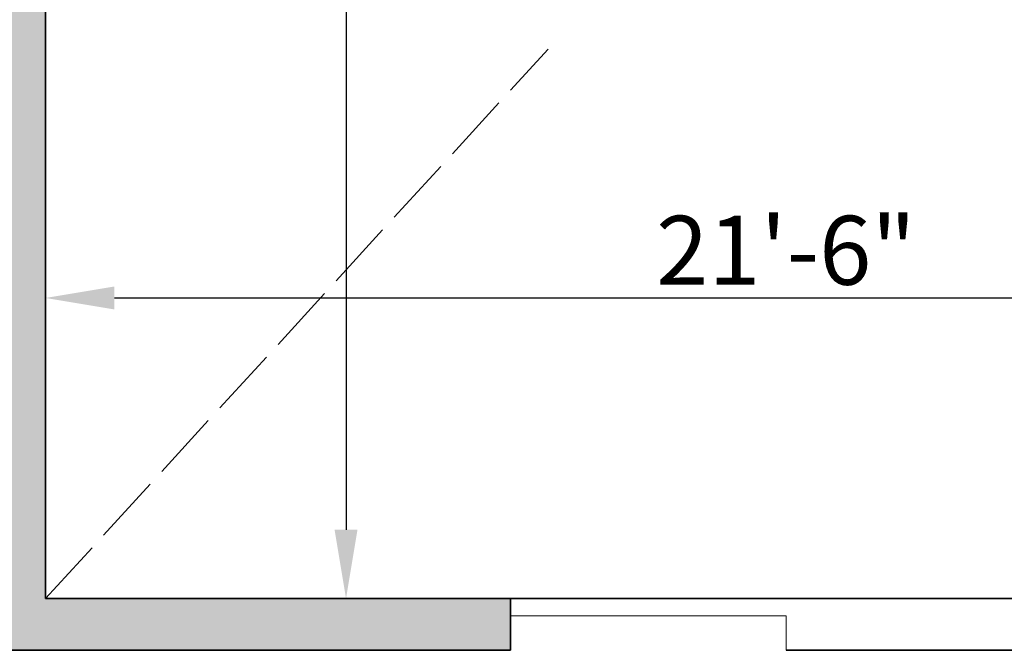
# Model space of a CAD drawing. Units: inches. Extents: x 2083 to 3317, y 1141 to 2115.
# Tile 108 of 256: x 2600 to 2772, y 1412 to 1522. Entities that reach past the tile are written whole.
import ezdxf

# ---------------------------------------------------------------- set-up
doc = ezdxf.new("R2010")
doc.units = ezdxf.units.IN
doc.linetypes.add('ACAD_ISO02W100', pattern=[15, 12, -3])
for name, color, linetype, lineweight in [('A-ANNO-DIMS', 2, 'Continuous', 18), ('A-FLOR-OPEN', 8, 'ACAD_ISO02W100', 13), ('A-GLAZ', 4, 'Continuous', 18), ('A-WALL', 7, 'Continuous', 35)]:
    doc.layers.add(name, color=color, linetype=linetype, lineweight=lineweight)
doc.layers.add('A-WALL-PATT', color=251, linetype='Continuous', lineweight=13, true_color=0x636466)
doc.styles.get("Standard").update_dxf_attribs({"font": 'arial.ttf'})
doc.dimstyles.new('ISO-25', dxfattribs={"dimtxt": 12, "dimasz": 12, "dimexe": 1.25, "dimexo": 0.625, "dimtad": 1, "dimlunit": 3, "dimtxsty": 'Standard', "dimcen": 2.5, "dimadec": 0, "dimazin": 0, "dimtfac": 1, "dimtmove": 0, "dimatfit": 3, "dimfxl": 1, "dimarcsym": 0})

# ---------------------------------------------------------------- blocks, each defined once
blk = doc.blocks.new('*D43')
at = {"layer": 'A-ANNO-DIMS', "color": 0, "lineweight": -2, "transparency": 16777216}
for p, q in [((2604.96, 1421.39), (2604.96, 1474.36)), ((2862.96, 1421.39), (2862.96, 1474.36)), ((2616.96, 1473.11), (2850.96, 1473.11))]:
    blk.add_line(p, q, dxfattribs=at)
at = {"layer": 'A-ANNO-DIMS', "color": 0, "transparency": 16777216}
for points in [[(2616.96, 1475.11), (2616.96, 1471.11), (2604.96, 1473.11)], [(2850.96, 1475.11), (2850.96, 1471.11), (2862.96, 1473.11)]]:
    blk.add_solid(points, dxfattribs=at)
at = {"layer": 'Defpoints', "color": 0, "transparency": 16777216}
for p in [(2862.96, 1473.11), (2604.96, 1420.76), (2862.96, 1420.76)]:
    blk.add_point(p, dxfattribs=at)
at = {"layer": 'A-ANNO-DIMS', "color": 0, "transparency": 16777216, "insert": (2733.96, 1479.86), "char_height": 12, "attachment_point": 5}
blk.add_mtext('21\'-6"', dxfattribs=at)
blk = doc.blocks.new('*D44')
at = {"layer": 'A-ANNO-DIMS', "color": 0, "lineweight": -2, "transparency": 16777216}
for p, q in [((2605.58, 1702.76), (2658.56, 1702.76)), ((2657.31, 1690.76), (2657.31, 1432.76)), ((2605.58, 1420.76), (2658.56, 1420.76))]:
    blk.add_line(p, q, dxfattribs=at)
at = {"layer": 'A-ANNO-DIMS', "color": 0, "transparency": 16777216}
for points in [[(2655.31, 1690.76), (2659.31, 1690.76), (2657.31, 1702.76)], [(2655.31, 1432.76), (2659.31, 1432.76), (2657.31, 1420.76)]]:
    blk.add_solid(points, dxfattribs=at)
at = {"layer": 'Defpoints', "color": 0, "transparency": 16777216}
for p in [(2604.96, 1702.76), (2604.96, 1420.76), (2657.31, 1420.76)]:
    blk.add_point(p, dxfattribs=at)
at = {"layer": 'A-ANNO-DIMS', "color": 0, "transparency": 16777216, "insert": (2650.55, 1561.76), "char_height": 12, "attachment_point": 5, "rotation": 90}
blk.add_mtext('23\'-6"', dxfattribs=at)

msp = doc.modelspace()

# ---------------------------------------------------------------- hatches: boundary and pattern name
at = {"layer": 'A-WALL-PATT'}
h = msp.add_hatch(color=256, dxfattribs=at)
h.dxf.hatch_style = 1
h.paths.add_polyline_path([(3126.96, 2020.761), (2748.96, 2020.761), (2604.96, 2020.761), (2226.96, 2020.761), (2226.96, 1702.761), (2466.96, 1702.761), (2466.96, 1582.761), (2418.96, 1582.761), (2418.96, 1477.761), (2226.96, 1477.761), (2226.96, 1263.261), (2544.96, 1263.261), (2544.96, 1411.761), (2604.96, 1411.761), (2685.96, 1411.761), (2685.96, 1420.761), (2604.96, 1420.761), (2604.96, 1573.761), (2604.96, 1702.761), (2604.96, 2011.761), (2748.96, 2011.761), (2748.96, 1702.761), (2862.96, 1702.761), (2862.96, 1621.761), (2871.96, 1621.761), (2871.96, 1702.761), (2883.96, 1702.761), (2883.96, 1706.939, -0.0264593), (2883.96, 1711.761), (2757.96, 1711.761), (2757.96, 1807.761), (2787.96, 1807.761), (2787.96, 1812.261), (2757.96, 1812.261), (2757.96, 2011.761), (2877.96, 2011.761), (2877.96, 1812.261), (2847.96, 1812.261), (2847.96, 1807.761), (2889.836, 1807.761), (2889.836, 1812.261), (2882.46, 1812.261), (2882.46, 2011.761), (3117.96, 2011.761), (3117.96, 1812.261), (2937.836, 1812.261), (2937.836, 1807.761), (2995.71, 1807.761), (2995.71, 1796.118), (3000.21, 1796.118), (3000.21, 1807.761), (3117.96, 1807.761), (3117.96, 1711.761), (3000.21, 1711.761), (3000.21, 1760.118), (2998.573, 1760.118, -0.020711), (2995.71, 1760.118), (2995.71, 1711.761), (2931.96, 1711.761), (2931.96, 1702.761), (3126.96, 1702.761)])
h.paths.add_polyline_path([(2471.46, 2011.761), (2471.46, 1810.011), (2462.717, 1810.011), (2462.717, 1805.511), (2505.96, 1805.511), (2505.96, 1810.011), (2475.96, 1810.011), (2475.96, 2011.761), (2595.96, 2011.761), (2595.96, 1810.011), (2565.96, 1810.011), (2565.96, 1805.511), (2595.96, 1805.511), (2595.96, 1711.761), (2235.96, 1711.761), (2235.96, 1805.511), (2353.71, 1805.511), (2353.71, 1796.054), (2358.21, 1796.054), (2358.21, 1805.511), (2414.717, 1805.511), (2414.717, 1810.011), (2235.96, 1810.011), (2235.96, 2011.761)], flags=16)
h.paths.add_polyline_path([(2270.205, 1994.61), (2270.205, 1970.61), (2246.205, 1970.61), (2246.205, 1994.61)], flags=0)
edge = h.paths.add_edge_path(flags=0)
edge.add_ellipse((2332.027, 1899.798), major_axis=(-3.043, 3.043), ratio=0.1682525, start_angle=-161.33217, end_angle=-156.30711, ccw=False)
edge.add_ellipse((2333.082, 1898.744), major_axis=(-1.055, 1.055), ratio=0.4535321, start_angle=-123.37102, end_angle=-94.15911)
edge = h.paths.add_edge_path(flags=0)
edge.add_ellipse((2332.027, 1968.876), major_axis=(3.043, 3.043), ratio=0.1682525, start_angle=18.66783, end_angle=23.69289)
edge.add_spline(control_points=[(2332.926, 1970.691), (2332.227, 1970.336), (2330.894, 1969.659), (2328.413, 1970.932), (2327.204, 1967.749), (2324.71, 1969.956), (2322.533, 1967.012), (2320.013, 1971.296), (2317.68, 1968.158), (2316.041, 1967.102), (2315.427, 1966.81)], knot_values=[0, 0, 0, 0, 2.2670587, 4.3245589, 6.6855835, 8.8786411, 11.121502, 14.300359, 17.7552837, 19.732645, 19.732645, 19.732645, 19.732645], degree=3, periodic=0)
edge.add_ellipse((2332.027, 1968.876), major_axis=(3.043, 3.043), ratio=0.1682525, start_angle=18.66783, end_angle=23.69289, ccw=False)
edge.add_ellipse((2333.082, 1969.931), major_axis=(1.055, 1.055), ratio=0.4535321, start_angle=56.62898, end_angle=85.84089, ccw=False)
edge = h.paths.add_edge_path(flags=0)
edge.add_spline(control_points=[(2296.428, 1967.988), (2293.628, 1965.336), (2287.704, 1959.727), (2299.744, 1949.996), (2294.533, 1935.669), (2290.573, 1920.604), (2293.394, 1909.974), (2296.185, 1904.967)], knot_values=[0.0991853, 0.0991853, 0.0991853, 0.0991853, 0.3453009, 0.6198217, 0.9826526, 1.3860932, 1.8105546, 1.8105546, 1.8105546, 1.8105546], degree=3, periodic=0)
edge.add_spline(control_points=[(2296.185, 1904.967), (2297.384, 1902.619), (2298.001, 1901.949), (2298.553, 1901.468)], knot_values=[0.0062457, 0.0062457, 0.0062457, 0.0062457, 0.0554759, 0.0554759, 0.0554759, 0.0554759], degree=3, periodic=0)
edge.add_spline(control_points=[(2298.553, 1901.468), (2297.259, 1900.923), (2295.225, 1900.232), (2293.06, 1900.614), (2292.101, 1900.788), (2292.09, 1900.791)], knot_values=[0.3128349, 0.3128349, 0.3128349, 0.3128349, 0.4017797, 0.4749867, 0.4759027, 0.4759027, 0.4759027, 0.4759027], degree=3, periodic=0)
edge.add_arc((2292.794, 1904.664), 3.937, 215.4209, 259.69818, ccw=False)
edge.add_spline(control_points=[(2289.585, 1902.382), (2289.477, 1902.535), (2289.368, 1902.688), (2289.261, 1902.841)], knot_values=[0.1028719, 0.1028719, 0.1028719, 0.1028719, 0.1168958, 0.1168958, 0.1168958, 0.1168958], degree=3, periodic=0)
edge.add_spline(control_points=[(2289.261, 1902.841), (2288.687, 1902.55), (2287.64, 1902.02), (2285.881, 1901.874), (2283.853, 1901.504), (2281.72, 1899.711), (2278.467, 1899.493), (2276.157, 1901.883), (2272.259, 1899.804), (2267.778, 1901.843), (2262.244, 1900.184), (2257.415, 1901.782), (2254.318, 1900.726), (2253.178, 1900.337)], knot_values=[0, 0, 0, 0, 1.9079767, 3.4771759, 5.261074, 7.9728515, 11.6802485, 13.7179214, 16.9395917, 22.789562, 27.5025027, 33.5952153, 37.1456181, 37.1456181, 37.1456181, 37.1456181], degree=3, periodic=0)
edge.add_line((2253.178, 1900.337), (2250.244, 1902.841))
edge.add_line((2250.244, 1902.841), (2250.244, 1965.833))
edge.add_line((2250.244, 1965.833), (2253.178, 1968.337))
edge.add_spline(control_points=[(2253.178, 1968.337), (2254.318, 1967.948), (2257.415, 1966.892), (2262.244, 1968.49), (2267.778, 1966.831), (2271.527, 1968.537), (2273.876, 1967.828), (2274.207, 1967.728)], knot_values=[0, 0, 0, 0, 0.0901802, 0.2449351, 0.3646438, 0.5132331, 0.5378548, 0.5378548, 0.5378548, 0.5378548], degree=3, periodic=0)
edge.add_arc((2274.353, 1963.793), 3.937, 72.05113, 92.12795, ccw=False)
edge.add_arc((2281.297, 1985.23), 18.596, 252.05113, 288.56572)
edge.add_arc((2292.317, 1956.029), 12.646, 71.02679, 113.77822, ccw=False)
edge = h.paths.add_edge_path(flags=0)
edge.add_spline(control_points=[(2274.899, 1951.856), (2275.066, 1951.617), (2275.233, 1951.377), (2275.398, 1951.136)], knot_values=[1.4099157, 1.4099157, 1.4099157, 1.4099157, 1.4315903, 1.4315903, 1.4315903, 1.4315903], degree=3, periodic=0)
edge.add_spline(control_points=[(2275.398, 1951.136), (2275.792, 1950.562), (2276.179, 1949.984), (2276.546, 1949.397)], knot_values=[1.3582378, 1.3582378, 1.3582378, 1.3582378, 1.4099157, 1.4099157, 1.4099157, 1.4099157], degree=3, periodic=0)
edge.add_line((2276.546, 1949.397), (2277.437, 1947.862))
edge.add_spline(control_points=[(2277.437, 1947.862), (2276.304, 1945.673), (2274.64, 1942.427), (2274.632, 1938.094), (2272.799, 1930.852), (2274.356, 1943.897), (2275.948, 1947.923), (2276.546, 1949.397)], knot_values=[0.0056315, 0.0056315, 0.0056315, 0.0056315, 0.1860139, 0.2660015, 0.3570872, 0.5963902, 0.7397317, 0.7397317, 0.7397317, 0.7397317], degree=3, periodic=0)
edge.add_spline(control_points=[(2276.546, 1949.397), (2276.179, 1949.984), (2275.792, 1950.562), (2275.398, 1951.136)], knot_values=[1.3582378, 1.3582378, 1.3582378, 1.3582378, 1.4099157, 1.4099157, 1.4099157, 1.4099157], degree=3, periodic=0)
edge.add_spline(control_points=[(2275.398, 1951.136), (2274.943, 1950.08), (2274.208, 1948.025), (2273.935, 1944.851), (2272.469, 1937.627), (2273.466, 1945.696), (2274.701, 1951.059), (2274.899, 1951.856)], knot_values=[0.1043639, 0.1043639, 0.1043639, 0.1043639, 0.1896363, 0.2696239, 0.3607096, 0.6000126, 0.6446217, 0.6446217, 0.6446217, 0.6446217], degree=3, periodic=0)
h.paths.add_polyline_path([(2269.168, 1963.128, -0.3575267), (2268.171, 1960.976, -0.0925607), (2268.171, 1939.436, -0.3575267), (2269.168, 1937.285, -0.3575267), (2267.016, 1938.282, -0.1647847), (2254.686, 1938.282, -0.3575267), (2252.534, 1937.285, -0.3575267), (2253.531, 1939.436, -0.0925607), (2253.531, 1960.976, -0.3575267), (2252.534, 1963.128, -0.3575267), (2254.686, 1962.131, -0.1647847), (2267.016, 1962.131, -0.3575267)], flags=0)
h.paths.add_polyline_path([(2248.874, 1967.802), (2248.874, 1957.028), (2249.458, 1957.028), (2249.458, 1911.647), (2248.874, 1911.647), (2248.874, 1900.873), (2246.512, 1900.873, 0.1973271), (2244.15, 1902.457), (2244.15, 1966.218, 0.1973271), (2246.512, 1967.802)], flags=0)
h.paths.add_polyline_path([(2269.168, 1931.389, -0.3575267), (2268.171, 1929.238, -0.0925607), (2268.171, 1907.698, -0.3575267), (2269.168, 1905.547, -0.3575267), (2267.016, 1906.544, -0.1647847), (2254.686, 1906.544, -0.3575267), (2252.534, 1905.547, -0.3575267), (2253.531, 1907.698, -0.0925607), (2253.531, 1929.238, -0.3575267), (2252.534, 1931.389, -0.3575267), (2254.686, 1930.392, -0.1647847), (2267.016, 1930.392, -0.3575267)], flags=0)
edge = h.paths.add_edge_path(flags=0)
edge.add_spline(control_points=[(2276.197, 1906.724), (2276.168, 1909.029), (2276.114, 1913.372), (2270.598, 1924.925), (2273.905, 1919.013), (2275.922, 1916.262), (2275.475, 1912.402), (2277.258, 1910.381), (2276.696, 1908.225), (2276.646, 1906.813), (2276.618, 1906.008)], knot_values=[0, 0, 0, 0, 8.6102597, 16.2212739, 18.8430575, 23.8048978, 27.4408283, 29.3561016, 31.2034776, 33.6506866, 33.6506866, 33.6506866, 33.6506866], degree=3, periodic=0)
edge.add_spline(control_points=[(2276.618, 1906.008), (2276.623, 1905.624), (2276.498, 1904.629), (2275.442, 1903.855), (2274.937, 1903.08), (2274.859, 1902.841)], knot_values=[0.1564884, 0.1564884, 0.1564884, 0.1564884, 0.1843975, 0.2313765, 0.2505985, 0.2505985, 0.2505985, 0.2505985], degree=3, periodic=0)
edge.add_line((2274.859, 1902.841), (2276.506, 1902.841))
edge.add_spline(control_points=[(2276.506, 1902.841), (2276.788, 1903.085), (2277.665, 1904.125), (2278.25, 1904.341), (2277.654, 1908.527), (2278.156, 1906.228), (2278.1, 1905.286), (2278.847, 1904.069), (2277.857, 1903.415), (2277.874, 1902.991), (2277.904, 1902.841)], knot_values=[0.0595743, 0.0595743, 0.0595743, 0.0595743, 0.0807529, 0.1037415, 0.1697201, 0.1760361, 0.2071372, 0.2404744, 0.2623409, 0.2736605, 0.2736605, 0.2736605, 0.2736605], degree=3, periodic=0)
edge.add_line((2277.904, 1902.841), (2280.03, 1902.841))
edge.add_spline(control_points=[(2280.03, 1902.841), (2279.888, 1903.088), (2279.499, 1903.982), (2280.152, 1905.939), (2278.104, 1909.658), (2279.762, 1907.185), (2280.328, 1904.875), (2280.485, 1903.49), (2281.463, 1903.249), (2281.758, 1902.936), (2281.834, 1902.841)], knot_values=[0.013856, 0.013856, 0.013856, 0.013856, 0.0348738, 0.0888667, 0.1078792, 0.1267378, 0.158714, 0.1937575, 0.2174868, 0.2267221, 0.2267221, 0.2267221, 0.2267221], degree=3, periodic=0)
edge.add_spline(control_points=[(2281.834, 1902.841), (2281.788, 1902.827), (2281.647, 1902.783), (2281.396, 1902.859), (2281.088, 1902.985), (2280.721, 1903.061), (2280.333, 1903.026), (2280.125, 1902.899), (2280.03, 1902.841)], knot_values=[0, 0, 0, 0, 0.1441304, 0.435517, 0.7492759, 1.1530457, 1.5483707, 1.878348, 1.878348, 1.878348, 1.878348], degree=3, periodic=0)
edge.add_line((2280.03, 1902.841), (2277.904, 1902.841))
edge.add_spline(control_points=[(2277.904, 1902.841), (2277.893, 1902.796), (2277.865, 1902.68), (2277.607, 1902.687), (2277.274, 1902.801), (2276.838, 1902.62), (2276.584, 1902.789), (2276.506, 1902.841)], knot_values=[0, 0, 0, 0, 0.1271885, 0.3261988, 0.6280094, 1.2435704, 1.5153306, 1.5153306, 1.5153306, 1.5153306], degree=3, periodic=0)
edge.add_line((2276.506, 1902.841), (2274.859, 1902.841))
edge.add_spline(control_points=[(2274.859, 1902.841), (2274.814, 1902.899), (2274.725, 1903.013), (2274.493, 1903.119), (2274.244, 1902.961), (2273.937, 1903.185), (2273.614, 1902.983), (2273.408, 1902.883), (2273.322, 1902.841)], knot_values=[0, 0, 0, 0, 0.2184302, 0.4369566, 0.6879766, 0.9903786, 1.3983955, 1.6918498, 1.6918498, 1.6918498, 1.6918498], degree=3, periodic=0)
edge.add_spline(control_points=[(2273.322, 1902.841), (2273.617, 1903.446), (2274.274, 1904.538), (2276.027, 1904.574), (2276.207, 1906.584), (2276.197, 1906.724)], knot_values=[0.0122268, 0.0122268, 0.0122268, 0.0122268, 0.0594721, 0.1062177, 0.134458, 0.134458, 0.134458, 0.134458], degree=3, periodic=0)
h.paths.add_polyline_path([(2270.776, 1897.79), (2270.776, 1873.79), (2246.776, 1873.79), (2246.776, 1897.79)], flags=0)
h.paths.add_polyline_path([(2353.71, 1760.005), (2353.71, 1760.054), (2358.21, 1760.054, -0.033729)], flags=0)
h.paths.add_polyline_path([(2321.819, 1737.529), (2341.995, 1737.529, -0.4142136), (2343.203, 1736.321), (2343.203, 1721.021, -0.4142136), (2341.995, 1719.813), (2321.819, 1719.813, -0.4142136), (2320.611, 1721.021), (2320.611, 1736.321, -0.4142136)], flags=0)
h.paths.add_polyline_path([(2324.235, 1736.321), (2339.579, 1736.321, -0.4142136), (2341.995, 1733.905), (2341.995, 1725.45, -0.4142136), (2339.579, 1723.034), (2333.681, 1723.034), (2333.845, 1722.045, -0.8706461), (2335.425, 1721.826, -0.767327), (2333.923, 1721.423), (2331.291, 1721.423, -0.767327), (2329.788, 1721.826, -0.8706461), (2331.368, 1722.045), (2331.533, 1723.034), (2324.235, 1723.034, -0.4142136), (2321.819, 1725.45), (2321.819, 1733.905, -0.4142136)], flags=0)
h.paths.add_polyline_path([(2570.484, 1928.615), (2589.684, 1928.615), (2590.169, 1928.615), (2590.169, 1904.993), (2570.484, 1904.993)], flags=0)
h.paths.add_polyline_path([(2574.447, 1927.264, -1), (2572.829, 1927.264, -1)], flags=0)
h.paths.add_polyline_path([(2573.09, 1926.941), (2573.925, 1927.776), (2574.148, 1927.553), (2573.313, 1926.718)], flags=0)
h.paths.add_polyline_path([(2578.779, 1919.73, -1), (2571.592, 1919.73, -1)], flags=0)
h.paths.add_polyline_path([(2578.385, 1919.73, -1), (2571.985, 1919.73, -1)], flags=0)
h.paths.add_polyline_path([(2331.596, 1729.476, -1), (2333.618, 1729.476, -1)], flags=0)
h.paths.add_polyline_path([(2578.034, 1927.264, -1), (2576.416, 1927.264, -1)], flags=0)
h.paths.add_polyline_path([(2576.689, 1927.531), (2576.912, 1927.754), (2577.747, 1926.919), (2577.524, 1926.696)], flags=0)
h.paths.add_polyline_path([(2578.139, 1909.86, -1), (2572.232, 1909.86, -1)], flags=0)
h.paths.add_polyline_path([(2577.745, 1909.86, -1), (2572.625, 1909.86, -1)], flags=0)
h.paths.add_polyline_path([(2583.798, 1927.264, -1), (2582.179, 1927.264, -1)], flags=0)
h.paths.add_polyline_path([(2582.719, 1927.754), (2583.554, 1926.919), (2583.331, 1926.696), (2582.496, 1927.531)], flags=0)
h.paths.add_polyline_path([(2582.496, 1927.531), (2582.719, 1927.754), (2583.554, 1926.919), (2583.331, 1926.696)], flags=0)
h.paths.add_polyline_path([(2587.739, 1920.53, -1), (2581.832, 1920.53, -1)], flags=0)
h.paths.add_polyline_path([(2587.345, 1920.53, -1), (2582.225, 1920.53, -1)], flags=0)
h.paths.add_polyline_path([(2587.385, 1927.264, -1), (2585.766, 1927.264, -1)], flags=0)
h.paths.add_polyline_path([(2586.082, 1926.98), (2586.917, 1927.815), (2587.14, 1927.593), (2586.305, 1926.758)], flags=0)
h.paths.add_polyline_path([(2588.379, 1910.66, -1), (2581.192, 1910.66, -1)], flags=0)
h.paths.add_polyline_path([(2587.985, 1910.66, -1), (2581.585, 1910.66, -1)], flags=0)
h.paths.add_polyline_path([(2417.168, 1729.478), (2437.344, 1729.478, -0.4142136), (2438.552, 1728.27), (2438.552, 1712.969, -0.4142136), (2437.344, 1711.761), (2417.168, 1711.761, -0.4142136), (2415.96, 1712.969), (2415.96, 1728.27, -0.4142136)], flags=0)
h.paths.add_polyline_path([(2419.584, 1728.27), (2434.928, 1728.27, -0.4142136), (2437.344, 1725.854), (2437.344, 1717.398, -0.4142136), (2434.928, 1714.983), (2429.029, 1714.983), (2429.194, 1713.994, -0.8706461), (2430.774, 1713.775, -0.767327), (2429.271, 1713.372), (2426.64, 1713.372, -0.767327), (2425.137, 1713.775, -0.8706461), (2426.717, 1713.994), (2426.882, 1714.983), (2419.584, 1714.983, -0.4142136), (2417.168, 1717.398), (2417.168, 1725.854, -0.4142136)], flags=0)
h.paths.add_polyline_path([(2419.584, 1728.27), (2434.928, 1728.27, -0.4142136), (2437.344, 1725.854), (2437.344, 1717.398, -0.4142136), (2434.928, 1714.983), (2429.029, 1714.983), (2428.358, 1719.009), (2427.553, 1719.009), (2426.882, 1714.983), (2419.584, 1714.983, -0.4142136), (2417.168, 1717.398), (2417.168, 1725.854, -0.4142136)], flags=0)
h.paths.add_polyline_path([(2426.944, 1721.425, -1), (2428.967, 1721.425, -1)], flags=0)
h.paths.add_polyline_path([(2475.96, 1702.761), (2595.96, 1702.761), (2595.96, 1582.761), (2475.96, 1582.761)], flags=16)
h.paths.add_polyline_path([(2427.96, 1573.761), (2595.96, 1573.761), (2595.96, 1468.761), (2595.96, 1420.761), (2384.46, 1420.761), (2384.46, 1468.761), (2427.96, 1468.761)], flags=16)
h.paths.add_polyline_path([(2379.96, 1468.761), (2379.96, 1420.761), (2235.96, 1420.761), (2235.96, 1468.761)], flags=16)
h.paths.add_polyline_path([(2317.816, 1466.696), (2337.992, 1466.696, -0.4142136), (2339.2, 1465.488), (2339.2, 1450.187, -0.4142136), (2337.992, 1448.979), (2317.816, 1448.979, -0.4142136), (2316.608, 1450.187), (2316.608, 1465.488, -0.4142136)], flags=0)
h.paths.add_polyline_path([(2320.232, 1465.488), (2335.576, 1465.488, -0.4142136), (2337.992, 1463.072), (2337.992, 1454.616, -0.4142136), (2335.576, 1452.2), (2329.677, 1452.2), (2329.842, 1451.212, -0.8706461), (2331.422, 1450.992, -0.767327), (2329.92, 1450.59), (2327.288, 1450.59, -0.767327), (2325.785, 1450.992, -0.8706461), (2327.365, 1451.212), (2327.53, 1452.2), (2320.232, 1452.2, -0.4142136), (2317.816, 1454.616), (2317.816, 1463.072, -0.4142136)], flags=0)
h.paths.add_polyline_path([(2320.232, 1465.488), (2335.576, 1465.488, -0.4142136), (2337.992, 1463.072), (2337.992, 1454.616, -0.4142136), (2335.576, 1452.2), (2329.677, 1452.2), (2329.006, 1456.227), (2328.201, 1456.227), (2327.53, 1452.2), (2320.232, 1452.2, -0.4142136), (2317.816, 1454.616), (2317.816, 1463.072, -0.4142136)], flags=0)
h.paths.add_polyline_path([(2327.593, 1458.643, -1), (2329.615, 1458.643, -1)], flags=0)
h.paths.add_polyline_path([(2244.412, 1433.34), (2241.921, 1433.34, -0.4142136), (2240.018, 1435.244), (2240.018, 1440.953, -0.4142105), (2241.921, 1442.856), (2244.412, 1442.856, -1.9764724)], flags=0)
h.paths.add_polyline_path([(2245.357, 1434.398, -0.4142136), (2245.357, 1441.799, -2.1440985)], flags=0)
h.paths.add_polyline_path([(2535.96, 1416.261), (2535.96, 1272.261), (2235.96, 1272.261), (2235.96, 1416.261)], flags=16)
h.paths.add_polyline_path([(2260.12, 1384.293), (2260.12, 1362.039), (2237.865, 1362.039), (2237.865, 1384.293)], flags=0)
edge = h.paths.add_edge_path(flags=0)
edge.add_line((2318.252, 1362.093), (2318.146, 1362.001))
edge.add_ellipse((2317.445, 1360.431), major_axis=(2.822, 2.822), ratio=0.1682525, start_angle=18.66783, end_angle=20.94813, ccw=False)
edge.add_ellipse((2318.423, 1361.409), major_axis=(0.978, 0.978), ratio=0.4535321, start_angle=56.62898, end_angle=70.2262, ccw=False)
edge = h.paths.add_edge_path(flags=0)
edge.add_line((2319.107, 1295.571), (2319.015, 1295.677))
edge.add_ellipse((2317.445, 1296.378), major_axis=(-2.822, 2.822), ratio=0.1682525, start_angle=-161.33217, end_angle=-159.05187, ccw=False)
edge.add_ellipse((2318.423, 1295.4), major_axis=(-0.978, 0.978), ratio=0.4535321, start_angle=-123.37102, end_angle=-109.7738)
edge = h.paths.add_edge_path(flags=0)
edge.add_spline(control_points=[(2284.21, 1301.17), (2284.581, 1300.445), (2284.891, 1299.892), (2285.16, 1299.461)], knot_values=[0.0390658, 0.0390658, 0.0390658, 0.0390658, 0.0554759, 0.0554759, 0.0554759, 0.0554759], degree=3, periodic=0)
edge.add_line((2285.16, 1299.461), (2284.21, 1301.17))
edge = h.paths.add_edge_path(flags=0)
edge.add_line((2280.412, 1297.298), (2283.37, 1297.036))
edge.add_line((2283.37, 1297.036), (2286.406, 1297.926))
edge.add_spline(control_points=[(2286.406, 1297.926), (2285.305, 1297.463), (2284.345, 1297.129), (2283.37, 1297.036)], knot_values=[0.3943688, 0.3943688, 0.3943688, 0.3943688, 0.4759027, 0.4759027, 0.4759027, 0.4759027], degree=3, periodic=0)
edge.add_spline(control_points=[(2283.37, 1297.036), (2283.281, 1297.028), (2282.316, 1296.957), (2281.313, 1297.134), (2280.423, 1297.296), (2280.412, 1297.298)], knot_values=[0.3128349, 0.3128349, 0.3128349, 0.3128349, 0.3202458, 0.3934528, 0.3943688, 0.3943688, 0.3943688, 0.3943688], degree=3, periodic=0)
edge = h.paths.add_edge_path(flags=0)
edge.add_line((2284.436, 1359.607), (2280.446, 1355.328))
edge.add_line((2280.446, 1355.328), (2279.58, 1351.018))
edge.add_line((2279.58, 1351.018), (2282.413, 1346.58))
edge.add_spline(control_points=[(2282.413, 1346.58), (2283.153, 1345.589), (2284.253, 1344.029), (2284.801, 1342.387), (2284.935, 1341.806)], knot_values=[1.2400982, 1.2400982, 1.2400982, 1.2400982, 1.3328922, 1.3827123, 1.3827123, 1.3827123, 1.3827123], degree=3, periodic=0)
edge.add_spline(control_points=[(2284.935, 1341.806), (2285.319, 1340.141), (2285.233, 1338.409), (2284.91, 1336.654)], knot_values=[1.0974841, 1.0974841, 1.0974841, 1.0974841, 1.2400982, 1.2400982, 1.2400982, 1.2400982], degree=3, periodic=0)
edge.add_spline(control_points=[(2284.91, 1336.654), (2284.587, 1334.899), (2284.027, 1333.12), (2283.463, 1331.361)], knot_values=[0.9548699, 0.9548699, 0.9548699, 0.9548699, 1.0974841, 1.0974841, 1.0974841, 1.0974841], degree=3, periodic=0)
edge.add_line((2283.463, 1331.361), (2281.89, 1326.153))
edge.add_line((2281.89, 1326.153), (2280.756, 1321.056))
edge.add_line((2280.756, 1321.056), (2280.299, 1316.002))
edge.add_line((2280.299, 1316.002), (2280.716, 1310.95))
edge.add_line((2280.716, 1310.95), (2282.028, 1305.972))
edge.add_line((2282.028, 1305.972), (2284.21, 1301.17))
edge.add_spline(control_points=[(2284.21, 1301.17), (2283.341, 1302.73), (2282.612, 1304.336), (2282.028, 1305.972)], knot_values=[0.0991853, 0.0991853, 0.0991853, 0.0991853, 0.2417994, 0.2417994, 0.2417994, 0.2417994], degree=3, periodic=0)
edge.add_spline(control_points=[(2282.028, 1305.972), (2281.444, 1307.608), (2281.005, 1309.273), (2280.716, 1310.95)], knot_values=[0.2417994, 0.2417994, 0.2417994, 0.2417994, 0.3844135, 0.3844135, 0.3844135, 0.3844135], degree=3, periodic=0)
edge.add_spline(control_points=[(2280.716, 1310.95), (2280.433, 1312.588), (2280.289, 1314.277), (2280.299, 1315.962), (2280.299, 1316.002)], knot_values=[0.3844135, 0.3844135, 0.3844135, 0.3844135, 0.5236467, 0.5270276, 0.5270276, 0.5270276, 0.5270276], degree=3, periodic=0)
edge.add_spline(control_points=[(2280.299, 1316.002), (2280.312, 1317.687), (2280.478, 1319.368), (2280.756, 1321.056)], knot_values=[0.5270276, 0.5270276, 0.5270276, 0.5270276, 0.6696417, 0.6696417, 0.6696417, 0.6696417], degree=3, periodic=0)
edge.add_spline(control_points=[(2280.756, 1321.056), (2281.035, 1322.744), (2281.426, 1324.44), (2281.89, 1326.153)], knot_values=[0.6696417, 0.6696417, 0.6696417, 0.6696417, 0.8122558, 0.8122558, 0.8122558, 0.8122558], degree=3, periodic=0)
edge.add_spline(control_points=[(2281.89, 1326.153), (2282.264, 1327.533), (2282.788, 1329.262), (2283.353, 1331.018), (2283.463, 1331.361)], knot_values=[0.8122558, 0.8122558, 0.8122558, 0.8122558, 0.9270873, 0.9548699, 0.9548699, 0.9548699, 0.9548699], degree=3, periodic=0)
edge.add_line((2283.463, 1331.361), (2284.91, 1336.654))
edge.add_line((2284.91, 1336.654), (2284.935, 1341.806))
edge.add_line((2284.935, 1341.806), (2282.413, 1346.58))
edge.add_spline(control_points=[(2282.413, 1346.58), (2281.275, 1348.104), (2280.078, 1349.57), (2279.58, 1351.018)], knot_values=[1.3827123, 1.3827123, 1.3827123, 1.3827123, 1.5253264, 1.5253264, 1.5253264, 1.5253264], degree=3, periodic=0)
edge.add_spline(control_points=[(2279.58, 1351.018), (2279.443, 1351.415), (2279.136, 1352.857), (2279.735, 1354.29), (2280.446, 1355.328)], knot_values=[1.5253264, 1.5253264, 1.5253264, 1.5253264, 1.564439, 1.6679405, 1.6679405, 1.6679405, 1.6679405], degree=3, periodic=0)
edge.add_spline(control_points=[(2280.446, 1355.328), (2281.426, 1356.758), (2282.931, 1358.183), (2284.436, 1359.607)], knot_values=[1.6679405, 1.6679405, 1.6679405, 1.6679405, 1.8105546, 1.8105546, 1.8105546, 1.8105546], degree=3, periodic=0)
edge.add_arc((2280.623, 1348.518), 11.726, 71.02679, 113.77822)
edge.add_arc((2270.405, 1375.595), 17.244, 252.05113, 288.56572, ccw=False)
edge.add_arc((2263.966, 1355.718), 3.651, 72.05113, 92.12795)
edge.add_arc((2263.966, 1355.718), 3.651, 92.12795, 177.98513)
edge.add_spline(control_points=[(2260.318, 1355.846), (2260.26, 1354.221), (2260.551, 1350.187), (2262.999, 1346.766), (2264.473, 1344.649)], knot_values=[1.4315903, 1.4315903, 1.4315903, 1.4315903, 1.5641438, 1.7706953, 1.7706953, 1.7706953, 1.7706953], degree=3, periodic=0)
edge.add_line((2264.473, 1344.649), (2264.936, 1343.983))
edge.add_spline(control_points=[(2263.801, 1340.248), (2263.843, 1340.514), (2264.067, 1341.756), (2264.513, 1343.002), (2264.935, 1343.981)], knot_values=[0.5365702, 0.5365702, 0.5365702, 0.5365702, 0.5593494, 0.6446217, 0.6446217, 0.6446217, 0.6446217], degree=3, periodic=0)
edge.add_spline(control_points=[(2264.935, 1343.981), (2265.118, 1343.715), (2265.299, 1343.448), (2265.477, 1343.179)], knot_values=[1.3840767, 1.3840767, 1.3840767, 1.3840767, 1.4099157, 1.4099157, 1.4099157, 1.4099157], degree=3, periodic=0)
edge.add_spline(control_points=[(2265.477, 1343.179), (2265.655, 1342.911), (2265.829, 1342.641), (2265.999, 1342.369)], knot_values=[1.3582378, 1.3582378, 1.3582378, 1.3582378, 1.3840767, 1.3840767, 1.3840767, 1.3840767], degree=3, periodic=0)
edge.add_line((2265.999, 1342.369), (2266.826, 1340.946))
edge.add_spline(control_points=[(2266.826, 1340.946), (2268.894, 1337.09), (2271.398, 1325.843), (2270.516, 1310.569), (2275.919, 1301.861), (2277.79, 1299.199)], knot_values=[0.1168958, 0.1168958, 0.1168958, 0.1168958, 0.4729873, 1.0509689, 1.3137934, 1.3137934, 1.3137934, 1.3137934], degree=3, periodic=0)
edge.add_spline(control_points=[(2277.79, 1299.199), (2277.839, 1299.128), (2277.889, 1299.057), (2277.94, 1298.987)], knot_values=[0.1098839, 0.1098839, 0.1098839, 0.1098839, 0.1168958, 0.1168958, 0.1168958, 0.1168958], degree=3, periodic=0)
edge.add_line((2277.94, 1298.987), (2277.789, 1299.199))
edge.add_spline(control_points=[(2277.789, 1299.199), (2277.257, 1298.929), (2276.286, 1298.438), (2275.039, 1298.334), (2274.383, 1298.239), (2274.215, 1298.209)], knot_values=[33.1218702, 33.1218702, 33.1218702, 33.1218702, 35.0290557, 36.5982549, 37.1448269, 37.1448269, 37.1448269, 37.1448269], degree=3, periodic=0)
edge.add_line((2274.215, 1298.209), (2273.073, 1297.893))
edge.add_spline(control_points=[(2273.073, 1297.893), (2272.323, 1297.58), (2271.039, 1296.511), (2269.248, 1296.226), (2268.423, 1296.375)], knot_values=[26.5325843, 26.5325843, 26.5325843, 26.5325843, 29.198919, 31.8391012, 31.8391012, 31.8391012, 31.8391012], degree=3, periodic=0)
edge.add_line((2268.423, 1296.375), (2263.879, 1297.458))
edge.add_spline(control_points=[(2263.879, 1297.458), (2263.556, 1297.359), (2261.86, 1296.839), (2260.239, 1297.282), (2258.933, 1297.516)], knot_values=[15.9195506, 15.9195506, 15.9195506, 15.9195506, 16.9395917, 21.2260675, 21.2260675, 21.2260675, 21.2260675], degree=3, periodic=0)
edge.add_line((2258.933, 1297.516), (2254.055, 1297.329))
edge.add_spline(control_points=[(2254.055, 1297.329), (2253.756, 1297.296), (2252.114, 1297.165), (2250.462, 1297.544), (2249.13, 1297.668)], knot_values=[5.3065169, 5.3065169, 5.3065169, 5.3065169, 6.2764352, 10.6130337, 10.6130337, 10.6130337, 10.6130337], degree=3, periodic=0)
edge.add_line((2249.13, 1297.668), (2244.332, 1296.878))
edge.add_line((2244.332, 1296.878), (2241.611, 1299.199))
edge.add_line((2241.611, 1299.199), (2241.611, 1357.609))
edge.add_line((2241.611, 1357.609), (2244.332, 1359.931))
edge.add_line((2244.332, 1359.931), (2252.729, 1359.543))
edge.add_spline(control_points=[(2252.729, 1359.543), (2252.871, 1359.546), (2253.306, 1359.548), (2253.74, 1359.514), (2254.032, 1359.482)], knot_values=[0.233291, 0.233291, 0.233291, 0.233291, 0.2449351, 0.2689274, 0.2689274, 0.2689274, 0.2689274], degree=3, periodic=0)
edge.add_line((2254.032, 1359.482), (2259.587, 1359.416))
edge.add_spline(control_points=[(2259.587, 1359.416), (2260.677, 1359.629), (2262.073, 1359.897), (2263.524, 1359.459), (2263.83, 1359.366)], knot_values=[0.4225164, 0.4225164, 0.4225164, 0.4225164, 0.5132331, 0.5378548, 0.5378548, 0.5378548, 0.5378548], degree=3, periodic=0)
edge.add_arc((2263.966, 1355.718), 3.651, 72.05113, 92.12795, ccw=False)
edge.add_arc((2270.405, 1375.595), 17.244, 252.05113, 288.56572)
edge.add_arc((2280.623, 1348.518), 11.726, 71.02679, 113.77822, ccw=False)
h.paths.add_polyline_path([(2240.341, 1359.435), (2240.341, 1349.444), (2240.882, 1349.444), (2240.882, 1307.365), (2240.341, 1307.365), (2240.341, 1297.374), (2238.15, 1297.374, 0.1973271), (2235.96, 1298.843), (2235.96, 1357.966, 0.1973271), (2238.15, 1359.435)], flags=0)
h.paths.add_polyline_path([(2259.158, 1355.101, -0.3575267), (2258.233, 1353.106, -0.0925607), (2258.233, 1333.133, -0.3575267), (2259.158, 1331.138, -0.3575267), (2257.163, 1332.062, -0.1647847), (2245.729, 1332.062, -0.3575267), (2243.735, 1331.138, -0.3575267), (2244.659, 1333.133, -0.0925607), (2244.659, 1353.106, -0.3575267), (2243.735, 1355.101, -0.3575267), (2245.729, 1354.176, -0.1647847), (2257.163, 1354.176, -0.3575267)], flags=0)
edge = h.paths.add_edge_path(flags=0)
edge.add_line((2265.999, 1342.369), (2266.826, 1340.946))
edge.add_line((2266.826, 1340.946), (2265.308, 1337.814))
edge.add_line((2265.308, 1337.814), (2264.358, 1334.653))
edge.add_line((2264.358, 1334.653), (2264.262, 1333.8))
edge.add_spline(control_points=[(2264.262, 1333.8), (2264.208, 1333.187), (2264.162, 1332.366), (2264.007, 1331.414), (2263.969, 1331.202)], knot_values=[0.4644442, 0.4644442, 0.4644442, 0.4644442, 0.5166905, 0.5316081, 0.5316081, 0.5316081, 0.5316081], degree=3, periodic=0)
edge.add_spline(control_points=[(2263.969, 1331.202), (2263.775, 1330.119), (2263.424, 1328.791), (2263.257, 1328.531), (2263.234, 1328.515)], knot_values=[0.3726816, 0.3726816, 0.3726816, 0.3726816, 0.4488497, 0.4644442, 0.4644442, 0.4644442, 0.4644442], degree=3, periodic=0)
edge.add_spline(control_points=[(2263.234, 1328.515), (2263.096, 1328.42), (2263.131, 1329.301), (2263.275, 1330.616)], knot_values=[0.2809191, 0.2809191, 0.2809191, 0.2809191, 0.3726816, 0.3726816, 0.3726816, 0.3726816], degree=3, periodic=0)
edge.add_spline(control_points=[(2263.275, 1330.616), (2263.419, 1331.93), (2263.672, 1333.677), (2263.97, 1335.315)], knot_values=[0.1891566, 0.1891566, 0.1891566, 0.1891566, 0.2809191, 0.2809191, 0.2809191, 0.2809191], degree=3, periodic=0)
edge.add_spline(control_points=[(2263.97, 1335.315), (2264.1, 1336.032), (2264.419, 1337.622), (2264.755, 1338.864), (2264.947, 1339.491)], knot_values=[0.097394, 0.097394, 0.097394, 0.097394, 0.1375775, 0.1891566, 0.1891566, 0.1891566, 0.1891566], degree=3, periodic=0)
edge.add_spline(control_points=[(2264.947, 1339.491), (2265.29, 1340.606), (2265.644, 1341.494), (2265.999, 1342.369)], knot_values=[0.0056315, 0.0056315, 0.0056315, 0.0056315, 0.097394, 0.097394, 0.097394, 0.097394], degree=3, periodic=0)
h.paths.add_polyline_path([(2259.158, 1325.671, -0.3575267), (2258.233, 1323.676, -0.0925607), (2258.233, 1303.703, -0.3575267), (2259.158, 1301.708, -0.3575267), (2257.163, 1302.633, -0.1647847), (2245.729, 1302.633, -0.3575267), (2243.735, 1301.708, -0.3575267), (2244.659, 1303.703, -0.0925607), (2244.659, 1323.676, -0.3575267), (2243.735, 1325.671, -0.3575267), (2245.729, 1324.747, -0.1647847), (2257.163, 1324.747, -0.3575267)], flags=0)
edge = h.paths.add_edge_path(flags=0)
edge.add_spline(control_points=[(2261.709, 1317.311), (2261.679, 1317.418), (2261.762, 1317.389), (2262.491, 1316.09), (2262.962, 1315.301)], knot_values=[14.9558607, 14.9558607, 14.9558607, 14.9558607, 16.2212739, 18.6948259, 18.6948259, 18.6948259, 18.6948259], degree=3, periodic=0)
edge.add_spline(control_points=[(2262.962, 1315.301), (2262.99, 1315.254), (2263.702, 1314.067), (2264.349, 1313.127), (2264.73, 1312.164)], knot_values=[18.6948259, 18.6948259, 18.6948259, 18.6948259, 18.8430575, 22.433791, 22.433791, 22.433791, 22.433791], degree=3, periodic=0)
edge.add_spline(control_points=[(2264.73, 1312.164), (2264.876, 1311.796), (2265.177, 1310.77), (2265.143, 1309.559), (2265.248, 1308.824)], knot_values=[22.433791, 22.433791, 22.433791, 22.433791, 23.8048978, 26.1727562, 26.1727562, 26.1727562, 26.1727562], degree=3, periodic=0)
edge.add_line((2265.248, 1308.824), (2265.851, 1307.172))
edge.add_spline(control_points=[(2265.851, 1307.172), (2266.065, 1306.822), (2266.384, 1306.332), (2266.424, 1305.781), (2266.42, 1305.611)], knot_values=[28.0625624, 28.0625624, 28.0625624, 28.0625624, 29.3561016, 29.9117214, 29.9117214, 29.9117214, 29.9117214], degree=3, periodic=0)
edge.add_spline(control_points=[(2266.42, 1305.611), (2266.416, 1305.433), (2266.394, 1305.25), (2266.365, 1305.066)], knot_values=[29.9117214, 29.9117214, 29.9117214, 29.9117214, 30.4978371, 30.4978371, 30.4978371, 30.4978371], degree=3, periodic=0)
edge.add_line((2266.365, 1305.066), (2266.066, 1302.136))
edge.add_spline(control_points=[(2266.066, 1302.136), (2266.071, 1301.78), (2265.998, 1301.2), (2265.663, 1300.759), (2265.509, 1300.586)], knot_values=[0.1564884, 0.1564884, 0.1564884, 0.1564884, 0.1843975, 0.2035434, 0.2035434, 0.2035434, 0.2035434], degree=3, periodic=0)
edge.add_line((2265.509, 1300.586), (2264.435, 1299.199))
edge.add_line((2264.435, 1299.199), (2265.962, 1299.199))
edge.add_line((2265.962, 1299.199), (2267.336, 1301.175))
edge.add_line((2267.336, 1301.175), (2267.312, 1301.986))
edge.add_spline(control_points=[(2267.312, 1301.986), (2267.261, 1302.862), (2267.16, 1303.737), (2267.271, 1303.326)], knot_values=[0.1262286, 0.1262286, 0.1262286, 0.1262286, 0.1666174, 0.1666174, 0.1666174, 0.1666174], degree=3, periodic=0)
edge.add_spline(control_points=[(2267.271, 1303.326), (2267.28, 1303.294), (2267.31, 1303.175), (2267.373, 1302.884), (2267.406, 1302.683), (2267.418, 1302.601)], knot_values=[0.1666174, 0.1666174, 0.1666174, 0.1666174, 0.1697201, 0.1760361, 0.1807647, 0.1807647, 0.1807647, 0.1807647], degree=3, periodic=0)
edge.add_spline(control_points=[(2267.744, 1300.988), (2267.688, 1301.151), (2267.481, 1301.657), (2267.484, 1302.145), (2267.418, 1302.601)], knot_values=[0.1807647, 0.1807647, 0.1807647, 0.1807647, 0.1937665, 0.2201389, 0.2201389, 0.2201389, 0.2201389], degree=3, periodic=0)
edge.add_line((2267.418, 1302.601), (2267.744, 1300.988))
edge.add_spline(control_points=[(2267.744, 1300.988), (2267.832, 1300.732), (2267.932, 1300.31), (2267.555, 1299.975), (2267.429, 1299.829)], knot_values=[0.2201389, 0.2201389, 0.2201389, 0.2201389, 0.2404744, 0.2548903, 0.2548903, 0.2548903, 0.2548903], degree=3, periodic=0)
edge.add_line((2267.429, 1299.829), (2267.258, 1299.199))
edge.add_line((2267.258, 1299.199), (2269.23, 1299.199))
edge.add_spline(control_points=[(2269.23, 1299.199), (2269.099, 1299.429), (2268.843, 1300.016), (2269.012, 1300.916), (2268.947, 1301.661)], knot_values=[0.013856, 0.013856, 0.013856, 0.013856, 0.0348738, 0.0670726, 0.0670726, 0.0670726, 0.0670726], degree=3, periodic=0)
edge.add_line((2268.947, 1301.661), (2268.432, 1303.603))
edge.add_spline(control_points=[(2268.432, 1303.603), (2268.176, 1304.192), (2267.596, 1305.251), (2268.041, 1304.623), (2268.251, 1304.282)], knot_values=[0.0901547, 0.0901547, 0.0901547, 0.0901547, 0.1078792, 0.1202891, 0.1202891, 0.1202891, 0.1202891], degree=3, periodic=0)
edge.add_spline(control_points=[(2268.251, 1304.282), (2268.361, 1304.105), (2269.058, 1302.918), (2269.383, 1301.59), (2269.521, 1300.776), (2269.575, 1300.556)], knot_values=[0.1202891, 0.1202891, 0.1202891, 0.1202891, 0.1267378, 0.158714, 0.1735056, 0.1735056, 0.1735056, 0.1735056], degree=3, periodic=0)
edge.add_line((2269.575, 1300.556), (2270.686, 1299.421))
edge.add_spline(control_points=[(2270.686, 1299.421), (2270.767, 1299.357), (2270.838, 1299.281), (2270.903, 1299.199)], knot_values=[0.2181597, 0.2181597, 0.2181597, 0.2181597, 0.2267221, 0.2267221, 0.2267221, 0.2267221], degree=3, periodic=0)
edge.add_line((2270.937, 1299.193), (2270.903, 1299.199))
edge.add_spline(control_points=[(2270.903, 1299.199), (2270.86, 1299.186), (2270.73, 1299.146), (2270.496, 1299.216), (2270.272, 1299.308), (2270.121, 1299.348), (2270.063, 1299.36)], knot_values=[0.939174, 0.939174, 0.939174, 0.939174, 1.0833044, 1.3746911, 1.6884499, 1.878348, 1.878348, 1.878348, 1.878348], degree=3, periodic=0)
edge.add_line((2270.063, 1299.36), (2269.23, 1299.199))
edge.add_line((2269.23, 1299.199), (2267.258, 1299.199))
edge.add_spline(control_points=[(2267.258, 1299.199), (2267.248, 1299.157), (2267.223, 1299.05), (2266.984, 1299.057), (2266.809, 1299.116), (2266.677, 1299.109), (2266.637, 1299.105)], knot_values=[0.7576653, 0.7576653, 0.7576653, 0.7576653, 0.8848538, 1.0838641, 1.3856747, 1.5153306, 1.5153306, 1.5153306, 1.5153306], degree=3, periodic=0)
edge.add_spline(control_points=[(2266.637, 1299.105), (2266.485, 1299.089), (2266.236, 1299.017), (2266.035, 1299.151), (2265.962, 1299.199)], knot_values=[0, 0, 0, 0, 0.4859051, 0.7576653, 0.7576653, 0.7576653, 0.7576653], degree=3, periodic=0)
edge.add_line((2265.962, 1299.199), (2264.435, 1299.199))
edge.add_line((2264.435, 1299.199), (2263.858, 1299.367))
edge.add_spline(control_points=[(2263.858, 1299.367), (2263.819, 1299.371), (2263.78, 1299.386), (2263.74, 1299.402)], knot_values=[0.8459249, 0.8459249, 0.8459249, 0.8459249, 0.9786272, 0.9786272, 0.9786272, 0.9786272], degree=3, periodic=0)
edge.add_line((2263.722, 1299.396), (2263.01, 1299.199))
edge.add_spline(control_points=[(2263.01, 1299.199), (2263.246, 1299.683), (2263.506, 1300.128), (2263.873, 1300.408)], knot_values=[0.0122268, 0.0122268, 0.0122268, 0.0122268, 0.0529705, 0.0529705, 0.0529705, 0.0529705], degree=3, periodic=0)
edge.add_spline(control_points=[(2263.873, 1300.408), (2263.932, 1300.453), (2264.084, 1300.553), (2264.255, 1300.624), (2264.36, 1300.665)], knot_values=[0.0529705, 0.0529705, 0.0529705, 0.0529705, 0.0594721, 0.0690861, 0.0690861, 0.0690861, 0.0690861], degree=3, periodic=0)
edge.add_line((2264.36, 1300.665), (2265.142, 1301.078))
edge.add_line((2265.142, 1301.078), (2265.676, 1302.8))
edge.add_line((2265.676, 1302.8), (2265.541, 1305.704))
edge.add_line((2265.541, 1305.704), (2264.803, 1309.328))
edge.add_line((2264.803, 1309.328), (2263.041, 1314.092))
edge.add_spline(control_points=[(2263.041, 1314.092), (2262.384, 1315.671), (2261.796, 1316.998), (2261.709, 1317.311)], knot_values=[11.2168955, 11.2168955, 11.2168955, 11.2168955, 14.9558607, 14.9558607, 14.9558607, 14.9558607], degree=3, periodic=0)
h.paths.add_polyline_path([(2871.96, 1416.261), (2895.91, 1416.261), (2895.91, 1420.761), (2871.96, 1420.761), (2871.96, 1501.761), (2862.96, 1501.761), (2862.96, 1420.761), (2805.96, 1420.761), (2805.96, 1411.761), (2862.96, 1411.761), (2862.96, 1263.261), (3126.96, 1263.261), (3126.96, 1411.761), (3126.96, 1486.761), (2943.96, 1486.761), (2943.96, 1477.761), (2967.86, 1477.761), (2967.86, 1420.761), (2943.91, 1420.761), (2943.91, 1416.261), (3117.96, 1416.261), (3117.96, 1420.761), (2972.36, 1420.761), (2972.36, 1477.761), (3117.96, 1477.761), (3117.96, 1420.761), (3117.96, 1272.261), (2871.96, 1272.261)], flags=0)
h.paths.add_polyline_path([(2457.126, 1485.943), (2527.603, 1485.943), (2527.603, 1537.636), (2457.126, 1537.636)], flags=8)
h.paths.add_polyline_path([(2481.005, 1609.982), (2590.766, 1609.982), (2590.766, 1682.003), (2481.005, 1682.003)], flags=8)
h.paths.add_polyline_path([(2483.085, 1729.127), (2553.562, 1729.127), (2553.562, 1780.82), (2483.085, 1780.82)], flags=8)

# ---------------------------------------------------------------- linework, layer by layer
at = {"layer": 'A-FLOR-OPEN'}
msp.add_line((2604.96, 1420.761), (2692.5, 1516.445), dxfattribs=at)
at = {"layer": 'A-GLAZ'}
for p, q in [((2685.96, 1417.761), (2733.96, 1417.761)), ((2733.96, 1417.761), (2733.96, 1411.761))]:
    msp.add_line(p, q, dxfattribs=at)
at = {"layer": 'A-WALL'}
for p, q in [((2604.96, 1573.761), (2604.96, 1420.761)), ((2604.96, 1420.761), (2862.96, 1420.761)), ((2685.96, 1420.761), (2685.96, 1411.761)), ((2544.96, 1411.761), (2604.96, 1411.761)), ((2604.96, 1411.761), (2685.96, 1411.761)), ((2733.96, 1411.761), (2862.96, 1411.761))]:
    msp.add_line(p, q, dxfattribs=at)

# ---------------------------------------------------------------- dimensions: what is measured, and where the dimension line sits
at = {"layer": 'A-ANNO-DIMS'}
dim = msp.add_linear_dim(base=(2657.31, 1420.761), p1=(2604.96, 1702.761), p2=(2604.96, 1420.761), angle=270, dimstyle='ISO-25', override={"dimdec": 1, "dimlfac": 1, "dimrnd": 0, "dimzin": 1, "dimdsep": 46, "dimlunit": 4, "dimfrac": 2}, dxfattribs=at)
dim.commit()
dim.dimension.update_dxf_attribs({"geometry": '*D44', "text_midpoint": (2650.554, 1561.761)})
dim = msp.add_linear_dim(base=(2862.96, 1473.111), p1=(2604.96, 1420.761), p2=(2862.96, 1420.761), dimstyle='ISO-25', override={"dimdec": 1, "dimlfac": 1, "dimrnd": 0, "dimzin": 1, "dimdsep": 46, "dimlunit": 4, "dimfrac": 2}, dxfattribs=at)
dim.commit()
dim.dimension.update_dxf_attribs({"geometry": '*D43', "text_midpoint": (2733.96, 1479.863)})

doc.saveas('drawing.dxf')
